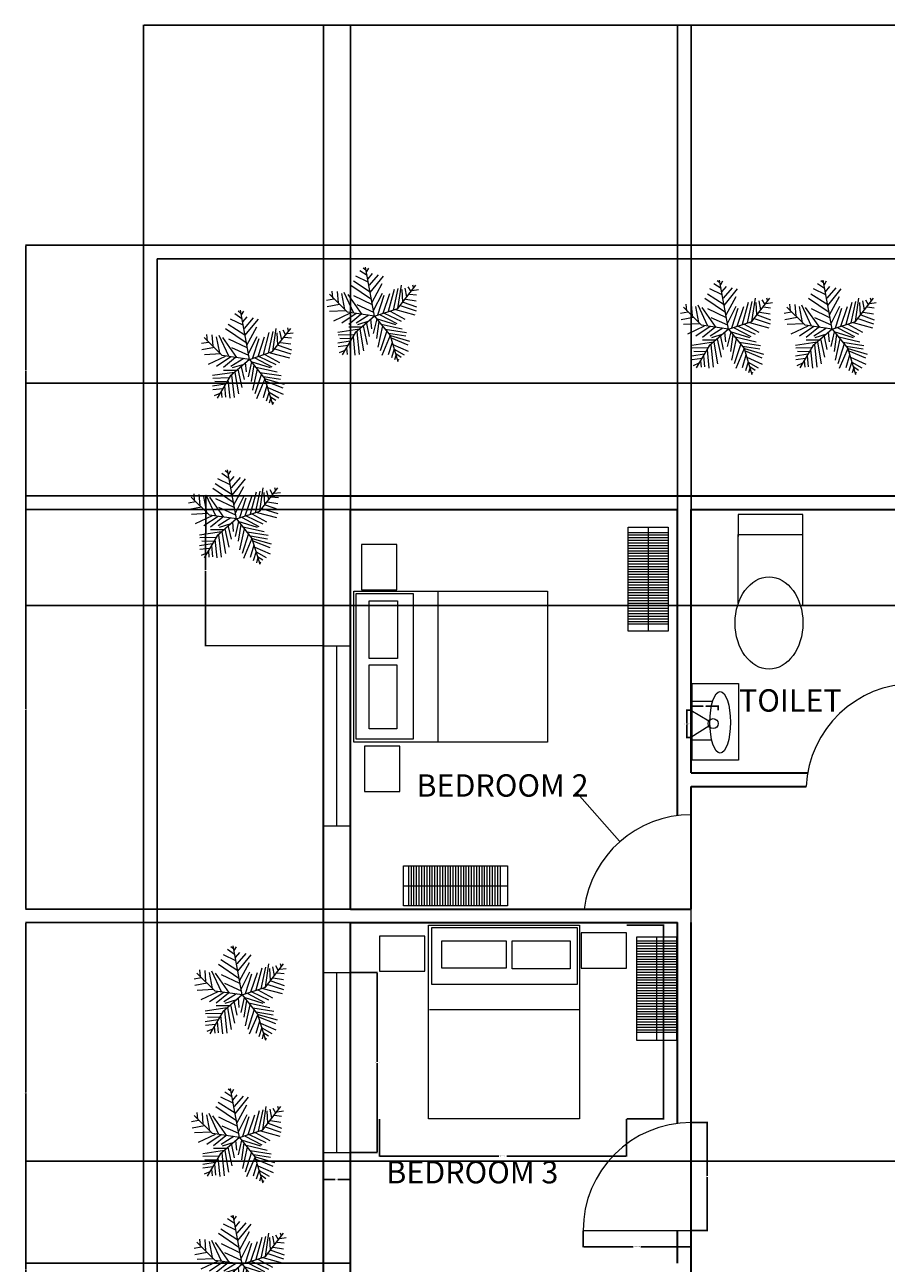
# Model space of a CAD drawing. Units: inches. Extents: x -86 to 773, y -188 to 560.
# Tile 2 of 6: x -86 to 201, y 147 to 560. Entities that reach past the tile are written whole.
import ezdxf

# ---------------------------------------------------------------- set-up
doc = ezdxf.new("R2010")
doc.units = ezdxf.units.IN
doc.header["$MEASUREMENT"] = 0
for name, color, linetype, lineweight in [('A-ANNO-DIMS', 2, 'Continuous', 18), ('A-AREA-IDEN', 7, 'Continuous', 25), ('A-DOOR', 7, 'Continuous', 18), ('A-FLOR-FIXT', 8, 'Continuous', 18), ('A-FURN', 8, 'Continuous', 18), ('A-FURN-PATT', 8, 'Continuous', 9), ('A-GLAZ', 7, 'Continuous', 18), ('A-WALL', 7, 'Continuous', 35), ('C-PROP', 7, 'Continuous', 25), ('L-PLNT-TREE', 8, 'Continuous', 9)]:
    doc.layers.add(name, color=color, linetype=linetype, lineweight=lineweight)
doc.styles.get("Standard").update_dxf_attribs({"font": 'arial.ttf'})
doc.dimstyles.get("Standard").update_dxf_attribs({"dimtxt": 0.18, "dimasz": 0.18, "dimexe": 0.18, "dimexo": 0.0625, "dimgap": 0.09, "dimtad": 0, "dimtih": 1, "dimtoh": 1, "dimdec": 4, "dimzin": 0, "dimdsep": 46, "dimtxsty": 'Standard', "dimcen": 0.09, "dimadec": 0, "dimazin": 0, "dimtfac": 1, "dimtdec": 4, "dimtofl": 0, "dimtmove": 0, "dimatfit": 3, "dimfxl": 1, "dimtolj": 1, "dimtzin": 0, "dimarcsym": 0})

# ---------------------------------------------------------------- blocks, each defined once
blk = doc.blocks.new('Trees - Metric')
for p, q in [((-185.1152, 1008.5578), (-553.1612, 1185.4942)), ((-221.9198, 1197.3052), (-433.5526, 1338.8594)), ((-258.7244, 1362.456), (-332.3336, 1421.4348)), ((0, 0), (-266.7, 1447.8)), ((-231.1146, 1315.2628), (-166.7002, 1421.4348)), ((-194.31, 1102.9442), (-65.4812, 1256.284)), ((-148.3106, 914.1968), (118.5418, 1220.9018)), ((-129.8956, 701.8528), (265.7602, 1185.4942)), ((-1234.059, 536.7274), (-1252.4486, 737.2604)), ((-93.091, 489.5342), (-700.3796, 902.3858)), ((-129.8956, 713.6638), (-626.7704, 1032.1544)), ((-74.7014, 418.7444), (219.7608, 961.39)), ((412.9786, 147.447), (587.8068, 796.2392)), ((560.197, 182.8292), (698.2206, 819.8358)), ((685.8, 228.6), (1219.2, 914.4)), ((689.0258, 230.0224), (790.2448, 914.1968)), ((808.6344, 784.4282), (827.0494, 418.7444)), ((891.4384, 831.6214), (946.658, 572.1096)), ((983.4626, 867.0036), (1066.2666, 725.4494)), ((1112.2914, 760.8316), (1296.3144, 784.4282)), ((1121.4862, 925.9824), (1149.0706, 831.6214)), ((-1206.4492, 501.3198), (-1418.082, 465.9376)), ((-800.1, 114.3), (-1333.5, 647.7)), ((-1105.2302, 725.4494), (-1077.6458, 395.1732)), ((-976.4268, 666.4706), (-884.4026, 194.6402)), ((-902.8176, 713.6638), (-617.5756, 100.2538)), ((-369.1382, 53.086), (-783.1836, 642.874)), ((-617.5756, 607.4918), (-74.7014, 347.98)), ((-28.6766, 171.0436), (228.9556, 678.2816)), ((100.1268, 41.275), (284.1498, 619.2774)), ((256.5654, 88.4682), (449.7832, 666.4706)), ((845.439, 418.7444), (1241.0948, 277.1902)), ((919.0482, 501.3198), (1222.6798, 454.152)), ((1029.462, 654.685), (1241.0948, 631.0884)), ((-1031.621, 347.98), (-1399.667, 277.1902)), ((-847.598, 159.2326), (-1326.0578, 135.636)), ((-718.7946, 88.4682), (-1215.644, -147.447)), ((-543.9664, 76.6572), (-967.2066, -206.4512)), ((0, 0), (-800.1, 114.3)), ((-405.9428, 53.086), (-764.794, -241.8334)), ((0, 0), (-571.5, -495.3)), ((-166.7002, 29.4894), (-543.9664, -206.4512)), ((-525.5514, 347.98), (-28.6766, 123.8504)), ((0, 0), (685.8, 228.6)), ((0, 0), (457.2, -571.5)), ((164.5412, 41.275), (661.416, -218.2368)), ((284.1498, 88.4682), (781.0246, -147.447)), ((458.978, 147.447), (891.4384, -88.4682)), ((615.4166, 194.6402), (1185.8752, 41.275)), ((753.4148, 312.5978), (1222.6798, 159.2326)), ((-387.5278, -324.4088), (-764.794, -324.4088)), ((-166.7002, -147.447), (-507.1618, -253.619)), ((-341.5284, -289.0012), (-221.9198, -831.6214)), ((-240.3094, -218.2368), (-157.5054, -595.7062)), ((-120.7008, -88.4682), (-93.091, -371.5766)), ((63.3222, -76.6826), (-37.8714, -513.1308)), ((44.9326, -64.897), (615.4166, -241.8334)), ((127.7366, -159.258), (54.1274, -654.685)), ((228.9556, -289.0012), (90.932, -914.1968)), ((192.151, -230.0224), (817.8292, -371.5766)), ((-442.7474, -383.3876), (-1086.8406, -477.7486)), ((-617.5756, -548.5384), (-1077.6458, -560.324)), ((-681.9646, -666.496), (-1022.4262, -654.685)), ((-571.5, -495.3), (-952.5, -1143)), ((-635.9652, -607.5172), (-580.771, -1150.1374)), ((-525.5514, -465.963), (-451.9422, -1126.5408)), ((-433.5526, -383.3876), (-323.1134, -1020.3688)), ((357.759, -430.5554), (164.5412, -1020.3688)), ((458.978, -572.1096), (210.5406, -1161.923)), ((311.7596, -383.3876), (937.4378, -477.7486)), ((412.9786, -501.3452), (919.0482, -583.9206)), ((457.2, -571.5), (685.8, -1333.5)), ((468.1982, -572.1096), (1029.462, -737.2604)), ((486.5878, -642.8994), (983.4626, -843.4324)), ((-718.7946, -737.2604), (-1086.8406, -796.2392)), ((-783.1836, -867.029), (-1077.6458, -902.4112)), ((-875.2078, -1008.5832), (-1040.8412, -1079.3476)), ((-829.2084, -937.7934), (-810.7934, -1126.5408)), ((-737.1842, -784.4536), (-709.5744, -1114.7298)), ((514.1976, -772.6426), (403.7838, -1138.3264)), ((578.612, -961.39), (495.7826, -1232.7128)), ((541.8074, -831.6214), (992.6574, -1032.1544)), ((578.612, -973.1756), (873.0488, -1138.3264)), ((624.6114, -1161.923), (587.8068, -1291.6916)), ((624.6114, -1102.9442), (781.0246, -1209.1162)), ((679.8056, -1268.095), (716.6102, -1291.6916))]:
    blk.add_line(p, q)
blk = doc.blocks.new('BED-DOUBLE-NIGHTSTANDS')
blk.add_line((16.69, 36.48), (66.76, 36.48))
for points in [[(16.43, 64.62), (66.76, 64.62), (66.76, 0), (16.43, 0)], [(17.47, 63.83), (65.98, 63.83), (65.98, 44.81), (17.47, 44.81)], [(82.41, 62.01), (67.29, 62.01), (67.29, 50.29), (82.41, 50.29)], [(15.13, 60.97), (0, 60.97), (0, 49.24), (15.13, 49.24)], [(20.86, 59.41), (42.25, 59.41), (42.25, 50.29), (20.86, 50.29)], [(44.34, 59.41), (63.63, 59.41), (63.63, 50.03), (44.34, 50.03)]]:
    blk.add_lwpolyline(points, close=True)
blk = doc.blocks.new('DOOR-LEAF-36')
blk.add_line((0, 0), (36, 0))
blk.add_arc((36, 0), 36, 90, 180)
blk = doc.blocks.new('WIN-60-W9')
for p, q in [((0, 60), (9, 60)), ((4.5, 60), (4.5, 0)), ((0, 0), (9, 0))]:
    blk.add_line(p, q)
blk = doc.blocks.new('BASIN-TAP')
blk.add_lwpolyline([(3.11, 5.27), (9.09, 9.11), (9.09, 0), (3.06, 3.55)])
blk.add_circle((1.66, 4.45), 1.66)
blk = doc.blocks.new('*D21')
at = {"layer": 'A-ANNO-DIMS', "color": 0, "lineweight": -2, "transparency": 16777216}
for p, q in [((32.08, 195.32), (32.08, 182.84)), ((114.5, 195.32), (114.5, 182.84)), ((32.26, 183.02), (71.98, 183.02)), ((114.32, 183.02), (74.6, 183.02))]:
    blk.add_line(p, q, dxfattribs=at)
at = {"layer": 'A-ANNO-DIMS', "color": 0, "transparency": 16777216}
for points in [[(32.26, 183.05), (32.26, 182.99), (32.08, 183.02)], [(114.32, 183.05), (114.32, 182.99), (114.5, 183.02)]]:
    blk.add_solid(points, dxfattribs=at)
at = {"layer": 'Defpoints', "color": 0, "transparency": 16777216}
for p in [(32.08, 195.38), (114.5, 195.38), (114.5, 183.02)]:
    blk.add_point(p, dxfattribs=at)
at = {"layer": 'A-ANNO-DIMS', "color": 0, "transparency": 16777216, "insert": (73.29, 183.02), "char_height": 0.18, "attachment_point": 5}
blk.add_mtext('\\A1;BED GROUP 82 TYP.', dxfattribs=at)
blk = doc.blocks.new('*D22')
at = {"layer": 'A-ANNO-DIMS', "color": 0, "lineweight": -2, "transparency": 16777216}
for p, q in [((114.56, 260), (127.04, 260)), ((126.86, 259.82), (126.86, 227.87)), ((126.86, 195.56), (126.86, 227.51)), ((114.56, 195.38), (127.04, 195.38))]:
    blk.add_line(p, q, dxfattribs=at)
at = {"layer": 'A-ANNO-DIMS', "color": 0, "transparency": 16777216}
for points in [[(126.83, 259.82), (126.89, 259.82), (126.86, 260)], [(126.83, 195.56), (126.89, 195.56), (126.86, 195.38)]]:
    blk.add_solid(points, dxfattribs=at)
at = {"layer": 'Defpoints', "color": 0, "transparency": 16777216}
for p in [(114.5, 260), (126.86, 260), (114.5, 195.38)]:
    blk.add_point(p, dxfattribs=at)
at = {"layer": 'A-ANNO-DIMS', "color": 0, "transparency": 16777216, "insert": (126.86, 227.69), "char_height": 0.18, "attachment_point": 5}
blk.add_mtext('\\A1;65 TYP.', dxfattribs=at)
blk = doc.blocks.new('*D23')
at = {"layer": 'A-ANNO-DIMS', "color": 0, "lineweight": -2, "transparency": 16777216}
for p, q in [((22.38, 244.22), (31.5, 244.22)), ((31.32, 244.04), (31.32, 214.4)), ((31.32, 184.4), (31.32, 214.03)), ((22.38, 184.22), (31.5, 184.22))]:
    blk.add_line(p, q, dxfattribs=at)
at = {"layer": 'A-ANNO-DIMS', "color": 0, "transparency": 16777216}
for points in [[(31.29, 244.04), (31.35, 244.04), (31.32, 244.22)], [(31.29, 184.4), (31.35, 184.4), (31.32, 184.22)]]:
    blk.add_solid(points, dxfattribs=at)
at = {"layer": 'Defpoints', "color": 0, "transparency": 16777216}
for p in [(22.32, 244.22), (31.32, 244.22), (22.32, 184.22)]:
    blk.add_point(p, dxfattribs=at)
at = {"layer": 'A-ANNO-DIMS', "color": 0, "transparency": 16777216, "insert": (31.32, 214.22), "char_height": 0.18, "attachment_point": 5}
blk.add_mtext('\\A1;WINDOW 60 TYP.', dxfattribs=at)
blk = doc.blocks.new('*D24')
at = {"layer": 'A-ANNO-DIMS', "color": 0, "lineweight": -2, "transparency": 16777216}
for p, q in [((13.32, 184.15), (13.32, 175.04)), ((22.32, 184.15), (22.32, 175.04)), ((13.5, 175.22), (17.36, 175.22)), ((22.14, 175.22), (18.27, 175.22))]:
    blk.add_line(p, q, dxfattribs=at)
at = {"layer": 'A-ANNO-DIMS', "color": 0, "transparency": 16777216}
for points in [[(13.5, 175.25), (13.5, 175.19), (13.32, 175.22)], [(22.14, 175.25), (22.14, 175.19), (22.32, 175.22)]]:
    blk.add_solid(points, dxfattribs=at)
at = {"layer": 'Defpoints', "color": 0, "transparency": 16777216}
for p in [(13.32, 184.22), (22.32, 184.22), (22.32, 175.22)]:
    blk.add_point(p, dxfattribs=at)
at = {"layer": 'A-ANNO-DIMS', "color": 0, "transparency": 16777216, "insert": (17.82, 175.22), "char_height": 0.18, "attachment_point": 5}
blk.add_mtext('\\A1;9 TYP.', dxfattribs=at)
blk = doc.blocks.new('*D31')
at = {"layer": 'A-ANNO-DIMS', "color": 0, "lineweight": -2, "transparency": 16777216}
for p, q in [((135.92, 331.65), (134.44, 331.65)), ((134.62, 331.47), (134.62, 327.28)), ((134.62, 322.72), (134.62, 326.91)), ((135.92, 322.54), (134.44, 322.54))]:
    blk.add_line(p, q, dxfattribs=at)
at = {"layer": 'A-ANNO-DIMS', "color": 0, "transparency": 16777216}
for points in [[(134.59, 331.47), (134.65, 331.47), (134.62, 331.65)], [(134.59, 322.72), (134.65, 322.72), (134.62, 322.54)]]:
    blk.add_solid(points, dxfattribs=at)
at = {"layer": 'Defpoints', "color": 0, "transparency": 16777216}
for p in [(135.98, 331.65), (134.62, 322.54), (135.98, 322.54)]:
    blk.add_point(p, dxfattribs=at)
at = {"layer": 'A-ANNO-DIMS', "color": 0, "transparency": 16777216, "insert": (134.62, 327.09), "char_height": 0.18, "attachment_point": 5}
blk.add_mtext('\\A1;BASIN TAP 9 TYP.', dxfattribs=at)
blk = doc.blocks.new('*D32')
at = {"layer": 'A-ANNO-DIMS', "color": 0, "lineweight": -2, "transparency": 16777216}
for p, q in [((135.98, 331.71), (135.98, 333.2)), ((136.16, 333.02), (140.07, 333.02)), ((144.89, 333.02), (140.98, 333.02)), ((145.07, 331.71), (145.07, 333.2))]:
    blk.add_line(p, q, dxfattribs=at)
at = {"layer": 'A-ANNO-DIMS', "color": 0, "transparency": 16777216}
for points in [[(136.16, 333.05), (136.16, 332.99), (135.98, 333.02)], [(144.89, 333.05), (144.89, 332.99), (145.07, 333.02)]]:
    blk.add_solid(points, dxfattribs=at)
at = {"layer": 'Defpoints', "color": 0, "transparency": 16777216}
for p in [(135.98, 333.02), (135.98, 331.65), (145.07, 331.65)]:
    blk.add_point(p, dxfattribs=at)
at = {"layer": 'A-ANNO-DIMS', "color": 0, "transparency": 16777216, "insert": (140.53, 333.02), "char_height": 0.18, "attachment_point": 5}
blk.add_mtext('\\A1;9 TYP.', dxfattribs=at)
blk = doc.blocks.new('*D35')
at = {"layer": 'A-ANNO-DIMS', "color": 0, "lineweight": -2, "transparency": 16777216}
for p, q in [((100.04, 158.13), (100.04, 152.61)), ((136.04, 158.13), (136.04, 152.61)), ((100.22, 152.79), (116.76, 152.79)), ((135.86, 152.79), (119.33, 152.79))]:
    blk.add_line(p, q, dxfattribs=at)
at = {"layer": 'A-ANNO-DIMS', "color": 0, "transparency": 16777216}
for points in [[(100.22, 152.82), (100.22, 152.76), (100.04, 152.79)], [(135.86, 152.82), (135.86, 152.76), (136.04, 152.79)]]:
    blk.add_solid(points, dxfattribs=at)
at = {"layer": 'Defpoints', "color": 0, "transparency": 16777216}
for p in [(100.04, 158.19), (136.04, 158.19), (136.04, 152.79)]:
    blk.add_point(p, dxfattribs=at)
at = {"layer": 'A-ANNO-DIMS', "color": 0, "transparency": 16777216, "insert": (118.04, 152.79), "char_height": 0.18, "attachment_point": 5}
blk.add_mtext('\\A1;DOOR LEAF 36 TYP.', dxfattribs=at)
blk = doc.blocks.new('*D36')
at = {"layer": 'A-ANNO-DIMS', "color": 0, "lineweight": -2, "transparency": 16777216}
for p, q in [((136.1, 194.19), (141.62, 194.19)), ((141.44, 194.01), (141.44, 176.37)), ((141.44, 158.37), (141.44, 176.01)), ((136.1, 158.19), (141.62, 158.19))]:
    blk.add_line(p, q, dxfattribs=at)
at = {"layer": 'A-ANNO-DIMS', "color": 0, "transparency": 16777216}
for points in [[(141.41, 194.01), (141.47, 194.01), (141.44, 194.19)], [(141.41, 158.37), (141.47, 158.37), (141.44, 158.19)]]:
    blk.add_solid(points, dxfattribs=at)
at = {"layer": 'Defpoints', "color": 0, "transparency": 16777216}
for p in [(136.04, 194.19), (141.44, 194.19), (136.04, 158.19)]:
    blk.add_point(p, dxfattribs=at)
at = {"layer": 'A-ANNO-DIMS', "color": 0, "transparency": 16777216, "insert": (141.44, 176.19), "char_height": 0.18, "attachment_point": 5}
blk.add_mtext('\\A1;36 TYP.', dxfattribs=at)
blk = doc.blocks.new('*D45')
at = {"layer": 'A-ANNO-DIMS', "color": 0, "lineweight": -2, "transparency": 16777216}
for p, q in [((-46.55, 486.72), (-46.55, 560.19)), ((-46.37, 560.01), (343.16, 560.01)), ((733.27, 560.01), (343.74, 560.01)), ((733.45, 486.72), (733.45, 560.19))]:
    blk.add_line(p, q, dxfattribs=at)
at = {"layer": 'A-ANNO-DIMS', "color": 0, "transparency": 16777216}
for points in [[(-46.37, 560.04), (-46.37, 559.98), (-46.55, 560.01)], [(733.27, 560.04), (733.27, 559.98), (733.45, 560.01)]]:
    blk.add_solid(points, dxfattribs=at)
at = {"layer": 'Defpoints', "color": 0, "transparency": 16777216}
for p in [(733.45, 560.01), (-46.55, 486.66), (733.45, 486.66)]:
    blk.add_point(p, dxfattribs=at)
at = {"layer": 'A-ANNO-DIMS', "color": 0, "transparency": 16777216, "insert": (343.45, 560.01), "char_height": 0.18, "attachment_point": 5}
blk.add_mtext('\\A1;780', dxfattribs=at)
blk = doc.blocks.new('*D51')
at = {"layer": 'A-ANNO-DIMS', "color": 0, "lineweight": -2, "transparency": 16777216}
for p, q in [((-46.61, 486.66), (-85.98, 486.66)), ((-85.8, 486.48), (-85.8, 445.07)), ((-85.8, 403.3), (-85.8, 444.71)), ((13.39, 403.12), (-85.98, 403.12))]:
    blk.add_line(p, q, dxfattribs=at)
at = {"layer": 'A-ANNO-DIMS', "color": 0, "transparency": 16777216}
for points in [[(-85.83, 486.48), (-85.77, 486.48), (-85.8, 486.66)], [(-85.83, 403.3), (-85.77, 403.3), (-85.8, 403.12)]]:
    blk.add_solid(points, dxfattribs=at)
at = {"layer": 'Defpoints', "color": 0, "transparency": 16777216}
for p in [(-85.8, 486.66), (-46.55, 486.66), (13.45, 403.12)]:
    blk.add_point(p, dxfattribs=at)
at = {"layer": 'A-ANNO-DIMS', "color": 0, "transparency": 16777216, "insert": (-85.8, 444.89), "char_height": 0.18, "attachment_point": 5}
blk.add_mtext('\\A1;83.54', dxfattribs=at)
blk = doc.blocks.new('*D55')
at = {"layer": 'A-ANNO-DIMS', "color": 0, "lineweight": -2, "transparency": 16777216}
for p, q in [((450.97, 440.74), (-85.98, 440.74)), ((-85.8, 440.56), (-85.8, 403.81)), ((-85.8, 366.7), (-85.8, 403.45)), ((450.97, 366.52), (-85.98, 366.52))]:
    blk.add_line(p, q, dxfattribs=at)
at = {"layer": 'A-ANNO-DIMS', "color": 0, "transparency": 16777216}
for points in [[(-85.83, 440.56), (-85.77, 440.56), (-85.8, 440.74)], [(-85.83, 366.7), (-85.77, 366.7), (-85.8, 366.52)]]:
    blk.add_solid(points, dxfattribs=at)
at = {"layer": 'Defpoints', "color": 0, "transparency": 16777216}
for p in [(451.03, 440.74), (-85.8, 366.52), (451.03, 366.52)]:
    blk.add_point(p, dxfattribs=at)
at = {"layer": 'A-ANNO-DIMS', "color": 0, "transparency": 16777216, "insert": (-85.8, 403.63), "char_height": 0.18, "attachment_point": 5}
blk.add_mtext('\\A1;74.22', dxfattribs=at)
blk = doc.blocks.new('*D56')
at = {"layer": 'A-ANNO-DIMS', "color": 0, "lineweight": -2, "transparency": 16777216}
for p, q in [((13.45, 403.19), (13.45, 560.19)), ((13.63, 560.01), (113.71, 560.01)), ((214.57, 560.01), (114.5, 560.01)), ((214.75, 403.19), (214.75, 560.19))]:
    blk.add_line(p, q, dxfattribs=at)
at = {"layer": 'A-ANNO-DIMS', "color": 0, "transparency": 16777216}
for points in [[(13.63, 560.04), (13.63, 559.98), (13.45, 560.01)], [(214.57, 560.04), (214.57, 559.98), (214.75, 560.01)]]:
    blk.add_solid(points, dxfattribs=at)
at = {"layer": 'Defpoints', "color": 0, "transparency": 16777216}
for p in [(214.75, 560.01), (13.45, 403.12), (214.75, 403.12)]:
    blk.add_point(p, dxfattribs=at)
at = {"layer": 'A-ANNO-DIMS', "color": 0, "transparency": 16777216, "insert": (114.1, 560.01), "char_height": 0.18, "attachment_point": 5}
blk.add_mtext('\\A1;201.3', dxfattribs=at)
blk = doc.blocks.new('*D57')
at = {"layer": 'A-ANNO-DIMS', "color": 0, "lineweight": -2, "transparency": 16777216}
for p, q in [((22.45, 398.69), (22.45, 560.19)), ((22.63, 560.01), (76.54, 560.01)), ((131.35, 560.01), (77.45, 560.01)), ((131.53, 398.69), (131.53, 560.19))]:
    blk.add_line(p, q, dxfattribs=at)
at = {"layer": 'A-ANNO-DIMS', "color": 0, "transparency": 16777216}
for points in [[(22.63, 560.04), (22.63, 559.98), (22.45, 560.01)], [(131.35, 560.04), (131.35, 559.98), (131.53, 560.01)]]:
    blk.add_solid(points, dxfattribs=at)
at = {"layer": 'Defpoints', "color": 0, "transparency": 16777216}
for p in [(131.53, 560.01), (22.45, 398.62), (131.53, 398.62)]:
    blk.add_point(p, dxfattribs=at)
at = {"layer": 'A-ANNO-DIMS', "color": 0, "transparency": 16777216, "insert": (76.99, 560.01), "char_height": 0.18, "attachment_point": 5}
blk.add_mtext('\\A1;109.08', dxfattribs=at)
blk = doc.blocks.new('*D58')
at = {"layer": 'A-ANNO-DIMS', "color": 0, "lineweight": -2, "transparency": 16777216}
for p, q in [((136.03, 398.69), (136.03, 560.19)), ((136.21, 560.01), (172.75, 560.01)), ((210.07, 560.01), (173.53, 560.01)), ((210.25, 398.69), (210.25, 560.19))]:
    blk.add_line(p, q, dxfattribs=at)
at = {"layer": 'A-ANNO-DIMS', "color": 0, "transparency": 16777216}
for points in [[(136.21, 560.04), (136.21, 559.98), (136.03, 560.01)], [(210.07, 560.04), (210.07, 559.98), (210.25, 560.01)]]:
    blk.add_solid(points, dxfattribs=at)
at = {"layer": 'Defpoints', "color": 0, "transparency": 16777216}
for p in [(210.25, 560.01), (136.03, 398.62), (210.25, 398.62)]:
    blk.add_point(p, dxfattribs=at)
at = {"layer": 'A-ANNO-DIMS', "color": 0, "transparency": 16777216, "insert": (173.14, 560.01), "char_height": 0.18, "attachment_point": 5}
blk.add_mtext('\\A1;74.22', dxfattribs=at)
blk = doc.blocks.new('*D59')
at = {"layer": 'A-ANNO-DIMS', "color": 0, "lineweight": -2, "transparency": 16777216}
for p, q in [((22.39, 398.62), (-85.98, 398.62)), ((-85.8, 398.44), (-85.8, 332.17)), ((-85.8, 265.54), (-85.8, 331.81)), ((22.39, 265.36), (-85.98, 265.36))]:
    blk.add_line(p, q, dxfattribs=at)
at = {"layer": 'A-ANNO-DIMS', "color": 0, "transparency": 16777216}
for points in [[(-85.83, 398.44), (-85.77, 398.44), (-85.8, 398.62)], [(-85.83, 265.54), (-85.77, 265.54), (-85.8, 265.36)]]:
    blk.add_solid(points, dxfattribs=at)
at = {"layer": 'Defpoints', "color": 0, "transparency": 16777216}
for p in [(22.45, 398.62), (-85.8, 265.36), (22.45, 265.36)]:
    blk.add_point(p, dxfattribs=at)
at = {"layer": 'A-ANNO-DIMS', "color": 0, "transparency": 16777216, "insert": (-85.8, 331.99), "char_height": 0.18, "attachment_point": 5}
blk.add_mtext('\\A1;133.26', dxfattribs=at)
blk = doc.blocks.new('*D60')
at = {"layer": 'A-ANNO-DIMS', "color": 0, "lineweight": -2, "transparency": 16777216}
for p, q in [((22.39, 260.86), (-85.98, 260.86)), ((-85.8, 260.68), (-85.8, 204.25)), ((-85.8, 147.46), (-85.8, 203.89)), ((22.39, 147.28), (-85.98, 147.28))]:
    blk.add_line(p, q, dxfattribs=at)
at = {"layer": 'A-ANNO-DIMS', "color": 0, "transparency": 16777216}
for points in [[(-85.83, 260.68), (-85.77, 260.68), (-85.8, 260.86)], [(-85.83, 147.46), (-85.77, 147.46), (-85.8, 147.28)]]:
    blk.add_solid(points, dxfattribs=at)
at = {"layer": 'Defpoints', "color": 0, "transparency": 16777216}
for p in [(22.45, 260.86), (-85.8, 147.28), (22.45, 147.28)]:
    blk.add_point(p, dxfattribs=at)
at = {"layer": 'A-ANNO-DIMS', "color": 0, "transparency": 16777216, "insert": (-85.8, 204.07), "char_height": 0.18, "attachment_point": 5}
blk.add_mtext('\\A1;113.58', dxfattribs=at)
blk = doc.blocks.new('*D73')
at = {"layer": 'A-ANNO-DIMS', "color": 0, "lineweight": -2, "transparency": 16777216}
for p, q in [((577.4, 181.27), (-85.98, 181.27)), ((-85.8, 181.09), (-85.8, 145.29)), ((-85.8, 109.12), (-85.8, 144.92)), ((577.4, 108.94), (-85.98, 108.94))]:
    blk.add_line(p, q, dxfattribs=at)
at = {"layer": 'A-ANNO-DIMS', "color": 0, "transparency": 16777216}
for points in [[(-85.83, 181.09), (-85.77, 181.09), (-85.8, 181.27)], [(-85.83, 109.12), (-85.77, 109.12), (-85.8, 108.94)]]:
    blk.add_solid(points, dxfattribs=at)
at = {"layer": 'Defpoints', "color": 0, "transparency": 16777216}
for p in [(-85.8, 181.27), (577.46, 181.27), (577.46, 108.94)]:
    blk.add_point(p, dxfattribs=at)
at = {"layer": 'A-ANNO-DIMS', "color": 0, "transparency": 16777216, "insert": (-85.8, 145.11), "char_height": 0.18, "attachment_point": 5}
blk.add_mtext('\\A1;72.33', dxfattribs=at)
blk = doc.blocks.new('*D88')
at = {"layer": 'A-ANNO-DIMS', "color": 0, "lineweight": -2, "transparency": 16777216}
for p, q in [((13.39, 403.12), (-25.98, 403.21)), ((-25.8, 403.03), (-25.85, 378.41)), ((-25.91, 353.43), (-25.86, 378.05)), ((13.28, 353.16), (-26.09, 353.25))]:
    blk.add_line(p, q, dxfattribs=at)
at = {"layer": 'A-ANNO-DIMS', "color": 0, "transparency": 16777216}
for points in [[(-25.83, 403.03), (-25.77, 403.03), (-25.8, 403.21)], [(-25.94, 353.43), (-25.88, 353.43), (-25.91, 353.25)]]:
    blk.add_solid(points, dxfattribs=at)
at = {"layer": 'Defpoints', "color": 0, "transparency": 16777216}
for p in [(-25.8, 403.21), (13.45, 403.12), (13.34, 353.16)]:
    blk.add_point(p, dxfattribs=at)
at = {"layer": 'A-ANNO-DIMS', "color": 0, "transparency": 16777216, "insert": (-25.86, 378.23), "char_height": 0.18, "attachment_point": 5}
blk.add_mtext('\\A1;49.96', dxfattribs=at)
blk = doc.blocks.new('*D94')
at = {"layer": 'A-ANNO-DIMS', "color": 0, "lineweight": -2, "transparency": 16777216}
for p, q in [((97.83, 304.03), (98.01, 304.03)), ((98.01, 304.03), (112.17, 287.96)), ((135.98, 260.8), (136.16, 260.8)), ((136.07, 260.71), (136.07, 260.89))]:
    blk.add_line(p, q, dxfattribs=at)
at = {"layer": 'A-ANNO-DIMS', "color": 0, "transparency": 16777216}
blk.add_solid([(112.19, 287.98), (112.14, 287.94), (112.29, 287.82)], dxfattribs=at)
at = {"layer": 'Defpoints', "color": 0, "transparency": 16777216}
for p in [(112.29, 287.82), (136.07, 260.8)]:
    blk.add_point(p, dxfattribs=at)
at = {"layer": 'A-ANNO-DIMS', "color": 0, "transparency": 16777216, "insert": (97.27, 304.03), "char_height": 0.18, "attachment_point": 5}
blk.add_mtext('\\A1;15X R36', dxfattribs=at)

msp = doc.modelspace()

# ---------------------------------------------------------------- hatches: boundary and pattern name
at = {"layer": 'A-FURN-PATT'}
h = msp.add_hatch(dxfattribs=at)
h.set_pattern_fill('ANSI31', color=256, scale=6.98128, angle=-45, style=0)
h.paths.add_polyline_path([(115.099, 360.2095), (128.3738, 360.2095), (128.3738, 391.6253), (115.099, 391.6253)])
h = msp.add_hatch(dxfattribs=at)
h.set_pattern_fill('ANSI31', color=256, scale=6.9813, angle=45, style=0)
h.paths.add_polyline_path([(41.1311, 266.4735), (72.5469, 266.4735), (72.5469, 279.7483), (41.1311, 279.7483)])
h = msp.add_hatch(dxfattribs=at)
h.set_pattern_fill('ANSI31', color=256, scale=6.9813, angle=-45, style=0)
h.paths.add_polyline_path([(117.8951, 223.718), (131.1699, 223.718), (131.1699, 255.1338), (117.8951, 255.1338)])

# ---------------------------------------------------------------- linework, layer by layer
at = {"layer": 'A-DOOR'}
for p, q in [((136.074, 260.8628), (136.074, 296.8024)), ((100.074, 260.8024), (131.5315, 260.8024)), ((136.0315, 260.8024), (136.074, 260.8024)), ((136.074, 260.8024), (136.074, 260.8628))]:
    msp.add_line(p, q, dxfattribs=at)
for centre, start, end in [((210.3869, 304.4977), 90, 177.176183), ((136.074, 260.8024), 90, 172.722267), ((136.074, 260.8024), 179.903794, 180)]:
    msp.add_arc(centre, 36, start, end, dxfattribs=at)
at = {"layer": 'A-FLOR-FIXT'}
for p, q in [((173.3341, 396.8849), (151.7345, 396.8849)), ((151.7345, 396.8849), (151.7345, 389.5723)), ((173.3341, 366.3625), (173.3341, 396.8849)), ((151.7345, 367.3163), (151.7345, 390.2082)), ((151.7345, 390.2082), (173.3341, 390.2082))]:
    msp.add_line(p, q, dxfattribs=at)
msp.add_lwpolyline([(136.353, 340.5575), (151.8148, 340.5575), (151.8148, 314.9952), (136.353, 314.9952)], close=True, dxfattribs=at)
msp.add_lwpolyline([(142.9365, 321.66), (136.3359, 321.66), (136.3359, 334.6652), (143.2322, 334.6652)], dxfattribs=at)
for centre, major_axis, ratio in [((162.0282, 360.7323), (0, 15.3922), 0.73614587), ((145.7374, 327.6207), (0, -10.2958), 0.33364881)]:
    msp.add_ellipse(centre, major_axis=major_axis, ratio=ratio, dxfattribs=at)
at = {"layer": 'A-FURN'}
for p, q in [((121.7364, 392.6396), (121.7364, 357.9905)), ((40.1168, 273.1109), (74.7659, 273.1109)), ((124.5325, 256.148), (124.5325, 221.4989))]:
    msp.add_line(p, q, dxfattribs=at)
for points in [[(128.3738, 357.9905), (115.099, 357.9905), (115.099, 392.6396), (128.3738, 392.6396)], [(74.7659, 279.7483), (74.7659, 266.4735), (40.1168, 266.4735), (40.1168, 279.7483)], [(131.1699, 221.4989), (117.8951, 221.4989), (117.8951, 256.148), (131.1699, 256.148)]]:
    msp.add_lwpolyline(points, close=True, dxfattribs=at)
at = {"layer": 'A-WALL'}
for p, q in [((13.4515, -143.4172), (13.4515, 403.1228)), ((13.4515, 403.1228), (214.7515, 403.1228)), ((22.4515, 398.6228), (131.5315, 398.6228)), ((22.4515, 265.3628), (22.4515, 398.6228)), ((131.5315, 296.5147), (131.5315, 398.6228)), ((136.0315, 398.6228), (210.2515, 398.6228)), ((136.0315, 310.7712), (136.0315, 398.6228)), ((136.0315, 310.7712), (174.9377, 310.7712)), ((136.0315, 306.2712), (174.4306, 306.2712)), ((136.0315, 265.3628), (136.0315, 306.2712)), ((22.4515, 265.3628), (136.074, 265.3628)), ((22.4515, 14.0228), (22.4515, 260.8628)), ((22.4515, 260.8628), (131.5315, 260.8628)), ((131.5315, 193.9077), (131.5315, 260.8628)), ((136.0315, 142.7828), (136.0315, 260.8628)), ((136.0315, 260.8628), (136.074, 260.8628)), ((131.5315, 147.2828), (131.5315, 158.1912))]:
    msp.add_line(p, q, dxfattribs=at)
at = {"layer": 'C-PROP'}
for p, q in [((-46.5485, -147.9172), (-46.5485, 486.6589)), ((-46.5485, 486.6589), (733.4515, 486.6589)), ((-42.0485, 482.1589), (728.9515, 482.1589)), ((-42.0485, -143.4172), (-42.0485, 482.1589)), ((-46.5485, -147.9172), (-46.5485, 403.1228))]:
    msp.add_line(p, q, dxfattribs=at)

# ---------------------------------------------------------------- block references
at = {"layer": 'A-DOOR'}
msp.add_blockref('DOOR-LEAF-36', (100.041, 158.191), dxfattribs=at)
at = {"layer": 'A-FLOR-FIXT', "rotation": 180}
msp.add_blockref('BASIN-TAP', (145.0693, 331.6486), dxfattribs=at)
at = {"layer": 'A-FURN', "rotation": 90.00000000000003}
msp.add_blockref('BED-DOUBLE-NIGHTSTANDS', (88.1475, 304.5403), dxfattribs=at)
at = {"layer": 'A-FURN'}
msp.add_blockref('BED-DOUBLE-NIGHTSTANDS', (32.084, 195.381), dxfattribs=at)
at = {"layer": 'A-GLAZ'}
for p in [(13.3379, 293.163), (13.3161, 184.2162)]:
    msp.add_blockref('WIN-60-W9', p, dxfattribs=at)
at = {"layer": 'L-PLNT-TREE', "xscale": 0.0112992005060107, "yscale": 0.0112992005060107, "zscale": 0.0112992005060107}
for p in [(30.4903, 463.0214), (148.5424, 458.7065), (183.0942, 458.7065), (-11.2599, 448.6384), (-15.5788, 395.4213), (-13.6777, 236.7263), (-14.5587, 189.1997), (-13.6777, 146.9538)]:
    msp.add_blockref('Trees - Metric', p, dxfattribs=at)

# ---------------------------------------------------------------- texts
at = {"layer": 'A-AREA-IDEN'}
for s, p in [('TOILET', (152.0366, 331.1867)), ('BEDROOM 2', (44.453, 302.8377)), ('BEDROOM 3', (34.3825, 173.9111))]:
    msp.add_text(s, height=7.45296, dxfattribs=at).set_placement(p)

# ---------------------------------------------------------------- dimensions: what is measured, and where the dimension line sits
at = {"layer": 'A-ANNO-DIMS'}
for base, p1, p2, override, picture, middle in [((733.4515, 560.0063), (-46.5485, 486.6589), (733.4515, 486.6589), {"dimdec": 0, "dimlfac": 1, "dimrnd": 0, "dimzin": 0, "dimdsep": 46, "dimlunit": 2}, '*D45', (343.4515, 560.0063)), ((214.7515, 560.0063), (13.4515, 403.1228), (214.7515, 403.1228), {"dimdec": 1, "dimlfac": 1, "dimrnd": 0, "dimzin": 0, "dimdsep": 46, "dimlunit": 2}, '*D56', (114.1015, 560.0063)), ((131.5315, 560.0063), (22.4515, 398.6228), (131.5315, 398.6228), {"dimdec": 2, "dimlfac": 1, "dimrnd": 0, "dimzin": 0, "dimdsep": 46, "dimlunit": 2}, '*D57', (76.9915, 560.0063)), ((210.2515, 560.0063), (136.0315, 398.6228), (210.2515, 398.6228), {"dimdec": 2, "dimlfac": 1, "dimrnd": 0, "dimzin": 0, "dimdsep": 46, "dimlunit": 2}, '*D58', (173.1415, 560.0063))]:
    dim = msp.add_linear_dim(base=base, p1=p1, p2=p2, dimstyle='Standard', override=override, dxfattribs=at)
    dim.commit()
    dim.dimension.update_dxf_attribs({"geometry": picture, "text_midpoint": middle})
for base, p1, p2, angle, picture, middle in [((-85.7985, 486.6589), (13.4515, 403.1228), (-46.5485, 486.6589), 90, '*D51', (-85.7985, 444.8909)), ((-85.7985, 366.5167), (451.0315, 440.7367), (451.0315, 366.5167), 90, '*D55', (-85.7985, 403.6267)), ((-25.7984, 403.2119), (13.3381, 353.1626), (13.4515, 403.1228), 89.870026, '*D88', (-25.8551, 378.2318)), ((-85.7985, 265.3628), (22.4515, 398.6228), (22.4515, 265.3628), 90, '*D59', (-85.7985, 331.9928)), ((-85.7985, 147.2828), (22.4515, 260.8628), (22.4515, 147.2828), 90, '*D60', (-85.7985, 204.0728)), ((-85.7985, 181.2736), (577.46, 108.94), (577.46, 181.2736), 90, '*D73', (-85.7985, 145.1068))]:
    dim = msp.add_linear_dim(base=base, p1=p1, p2=p2, angle=angle, dimstyle='Standard', override={"dimdec": 2, "dimlfac": 1, "dimrnd": 0, "dimzin": 0, "dimdsep": 46, "dimlunit": 2}, dxfattribs=at)
    dim.commit()
    dim.dimension.update_dxf_attribs({"geometry": picture, "text_midpoint": middle})
for base, p1, p2, angle, text, picture, middle in [((134.6161, 322.5373), (135.9827, 331.6484), (135.9827, 322.5373), 270, 'BASIN TAP <> TYP.', '*D31', (134.6161, 327.0928)), ((135.9827, 333.015), (145.069, 331.6484), (135.9827, 331.6484), 180, '<> TYP.', '*D32', (140.5259, 333.015)), ((126.8578, 259.9973), (114.496, 195.3809), (114.496, 259.9973), 90, '<> TYP.', '*D22', (126.8578, 227.6891)), ((31.3164, 244.2158), (22.3164, 184.2158), (22.3164, 244.2158), 90, 'WINDOW <> TYP.', '*D23', (31.3164, 214.2158)), ((141.4409, 194.1912), (136.0409, 158.1912), (136.0409, 194.1912), 90, '<> TYP.', '*D36', (141.4409, 176.1912))]:
    dim = msp.add_linear_dim(base=base, p1=p1, p2=p2, angle=angle, text=text, dimstyle='Standard', override={"dimdec": 0, "dimlfac": 1, "dimrnd": 0, "dimzin": 0, "dimdsep": 46, "dimlunit": 2}, dxfattribs=at)
    dim.commit()
    dim.dimension.update_dxf_attribs({"geometry": picture, "text_midpoint": middle})
dim = msp.add_radius_dim(center=(136.074, 260.8024), mpoint=(112.2853, 287.8227), text='15X <>', dimstyle='Standard', override={"dimdec": 0, "dimlfac": 1, "dimrnd": 0, "dimzin": 0, "dimdsep": 46, "dimlunit": 2}, dxfattribs=at)
dim.commit()
dim.dimension.update_dxf_attribs({"geometry": '*D94', "text_midpoint": (97.2722, 304.0349), "dimtype": 164})
for base, p1, p2, text, picture, middle in [((114.496, 183.0192), (32.0844, 195.3809), (114.496, 195.3809), 'BED GROUP <> TYP.', '*D21', (73.2902, 183.0192)), ((22.3164, 175.2158), (13.3164, 184.2158), (22.3164, 184.2158), '<> TYP.', '*D24', (17.8164, 175.2158)), ((136.0409, 152.7912), (100.0409, 158.1912), (136.0409, 158.1912), 'DOOR LEAF <> TYP.', '*D35', (118.0409, 152.7912))]:
    dim = msp.add_linear_dim(base=base, p1=p1, p2=p2, text=text, dimstyle='Standard', override={"dimdec": 0, "dimlfac": 1, "dimrnd": 0, "dimzin": 0, "dimdsep": 46, "dimlunit": 2}, dxfattribs=at)
    dim.commit()
    dim.dimension.update_dxf_attribs({"geometry": picture, "text_midpoint": middle})

doc.saveas('drawing.dxf')
